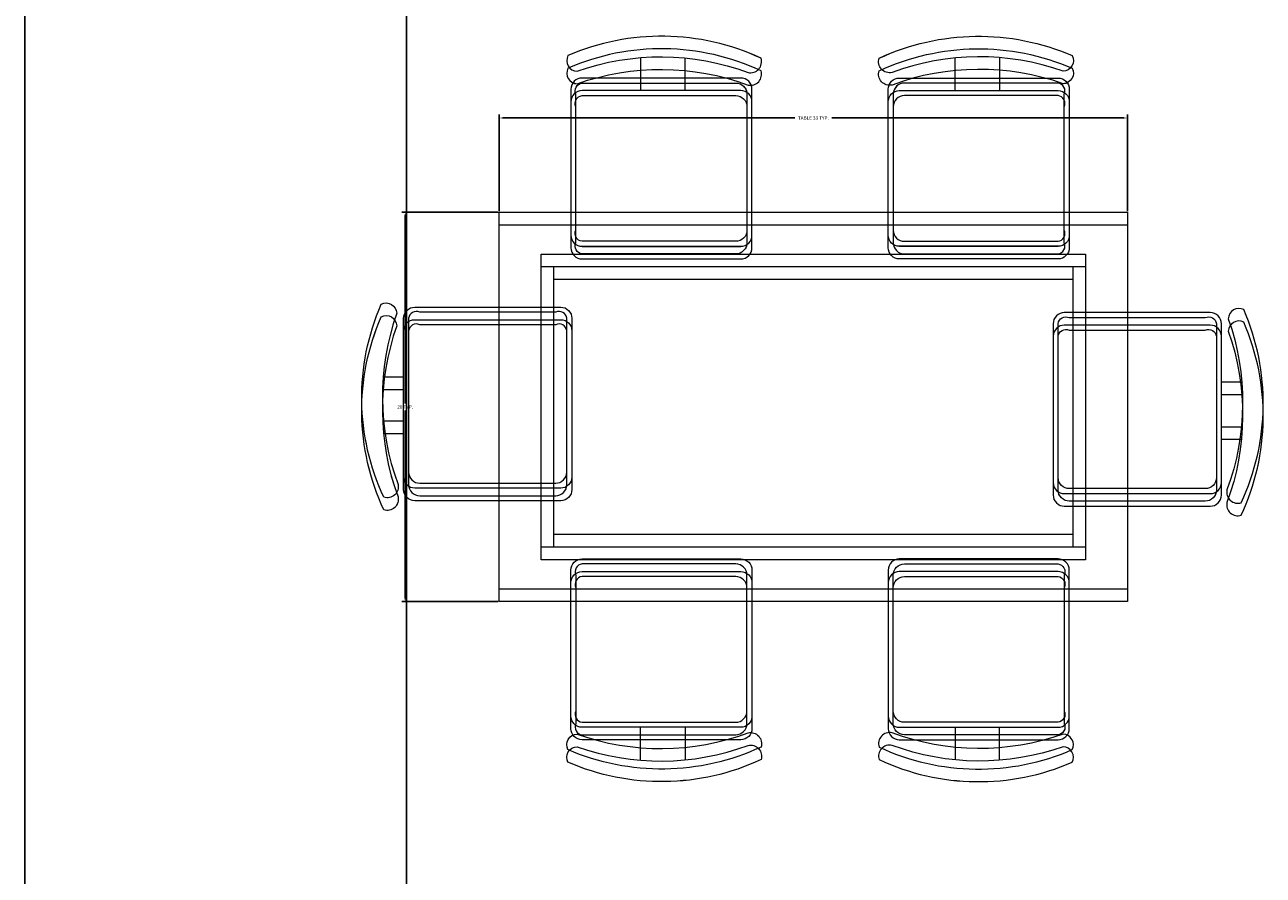
# Model space of a CAD drawing. Units: inches. Extents: x 1601 to 2297, y 1496 to 2631.
# Tile 52 of 57: x 2036 to 2100, y 2327 to 2371. Entities that reach past the tile are written whole.
import ezdxf

# ---------------------------------------------------------------- set-up
doc = ezdxf.new("R2010")
doc.units = ezdxf.units.IN
doc.layers.add('A-ANNO-DIMS', color=2, linetype='Continuous', lineweight=18)
doc.layers.add('A-FURN', color=8, linetype='Continuous', lineweight=18)
doc.styles.get("Standard").update_dxf_attribs({"font": 'arial.ttf'})
doc.dimstyles.get("Standard").update_dxf_attribs({"dimtxt": 0.18, "dimasz": 0.18, "dimexe": 0.18, "dimexo": 0.0625, "dimgap": 0.09, "dimtad": 0, "dimtih": 1, "dimtoh": 1, "dimdec": 4, "dimzin": 0, "dimdsep": 46, "dimtxsty": 'Standard', "dimcen": 0.09, "dimadec": 0, "dimazin": 0, "dimtfac": 1, "dimtdec": 4, "dimtofl": 0, "dimtmove": 0, "dimatfit": 3, "dimfxl": 1, "dimtolj": 1, "dimtzin": 0, "dimarcsym": 0})

# ---------------------------------------------------------------- blocks, each defined once
blk = doc.blocks.new('DINING-TABLE')
for points in [[(0, 20.416), (32.93, 20.416), (32.93, 0.659), (0, 0.659)], [(0, 20.416), (32.93, 20.416), (32.93, 0.658), (0, 0.658)], [(0, 20.416), (32.93, 20.416), (32.93, 0.659), (0, 0.659)], [(0, 20.416), (32.93, 20.416), (32.93, 0.658), (0, 0.658)], [(0, 19.758), (32.93, 19.758), (32.93, 0), (0, 0)], [(0, 19.758), (32.93, 19.758), (32.93, 0), (0, 0)], [(0, 19.758), (32.93, 19.758), (32.93, 0), (0, 0)], [(0, 19.758), (32.93, 19.758), (32.93, 0), (0, 0)], [(2.196, 18.221), (30.735, 18.221), (30.735, 2.854), (2.196, 2.854)], [(2.196, 18.221), (30.735, 18.221), (30.735, 2.854), (2.196, 2.854)], [(2.196, 18.221), (30.735, 18.221), (30.735, 2.854), (2.196, 2.854)], [(2.196, 18.221), (30.735, 18.221), (30.735, 2.854), (2.196, 2.854)], [(2.196, 17.563), (30.735, 17.563), (30.735, 2.195), (2.196, 2.195)], [(2.196, 17.563), (30.735, 17.563), (30.735, 2.195), (2.196, 2.195)], [(2.196, 17.562), (30.735, 17.562), (30.735, 2.195), (2.196, 2.195)], [(2.196, 17.562), (30.735, 17.562), (30.735, 2.195), (2.196, 2.195)], [(2.854, 17.563), (30.076, 17.563), (30.076, 3.513), (2.854, 3.513)], [(2.854, 17.563), (30.076, 17.563), (30.076, 3.513), (2.854, 3.513)], [(2.854, 17.562), (30.076, 17.562), (30.076, 3.512), (2.854, 3.512)], [(2.854, 17.562), (30.076, 17.562), (30.076, 3.512), (2.854, 3.512)], [(2.854, 16.904), (30.076, 16.904), (30.076, 2.854), (2.854, 2.854)], [(2.854, 16.904), (30.076, 16.904), (30.076, 2.854), (2.854, 2.854)], [(2.854, 16.904), (30.076, 16.904), (30.076, 2.854), (2.854, 2.854)], [(2.854, 16.904), (30.076, 16.904), (30.076, 2.854), (2.854, 2.854)]]:
    blk.add_lwpolyline(points, close=True)
blk = doc.blocks.new('*D16')
at = {"layer": 'A-ANNO-DIMS', "color": 0, "lineweight": -2, "transparency": 16777216}
for p, q in [((2060.42, 2361.732), (2060.42, 2366.789)), ((2060.6, 2366.609), (2075.922, 2366.609)), ((2093.17, 2366.609), (2077.849, 2366.609)), ((2093.35, 2361.732), (2093.35, 2366.789))]:
    blk.add_line(p, q, dxfattribs=at)
at = {"layer": 'A-ANNO-DIMS', "color": 0, "transparency": 16777216}
for points in [[(2060.6, 2366.639), (2060.6, 2366.579), (2060.42, 2366.609)], [(2093.17, 2366.639), (2093.17, 2366.579), (2093.35, 2366.609)]]:
    blk.add_solid(points, dxfattribs=at)
at = {"layer": 'Defpoints', "color": 0, "transparency": 16777216}
for p in [(2093.35, 2366.609), (2060.42, 2361.669), (2093.35, 2361.669)]:
    blk.add_point(p, dxfattribs=at)
at = {"layer": 'A-ANNO-DIMS', "color": 0, "transparency": 16777216, "insert": (2076.885, 2366.609), "char_height": 0.18, "attachment_point": 5}
blk.add_mtext('\\A1;TABLE 33 TYP.', dxfattribs=at)
blk = doc.blocks.new('*D17')
at = {"layer": 'A-ANNO-DIMS', "color": 0, "lineweight": -2, "transparency": 16777216}
for p, q in [((2060.358, 2361.669), (2055.301, 2361.669)), ((2055.481, 2361.489), (2055.481, 2351.643)), ((2055.481, 2341.433), (2055.481, 2351.279)), ((2060.358, 2341.253), (2055.301, 2341.253))]:
    blk.add_line(p, q, dxfattribs=at)
at = {"layer": 'A-ANNO-DIMS', "color": 0, "transparency": 16777216}
for points in [[(2055.451, 2361.489), (2055.511, 2361.489), (2055.481, 2361.669)], [(2055.451, 2341.433), (2055.511, 2341.433), (2055.481, 2341.253)]]:
    blk.add_solid(points, dxfattribs=at)
at = {"layer": 'Defpoints', "color": 0, "transparency": 16777216}
for p in [(2055.481, 2361.669), (2060.42, 2361.669), (2060.42, 2341.253)]:
    blk.add_point(p, dxfattribs=at)
at = {"layer": 'A-ANNO-DIMS', "color": 0, "transparency": 16777216, "insert": (2055.481, 2351.461), "char_height": 0.18, "attachment_point": 5}
blk.add_mtext('\\A1;20 TYP.', dxfattribs=at)
blk = doc.blocks.new('*D40')
at = {"layer": 'A-ANNO-DIMS', "color": 0, "lineweight": -2, "transparency": 16777216}
for p, q in [((2035.537, 1986.388), (2035.537, 2581.055)), ((2035.717, 2580.875), (2045.079, 2580.875)), ((2055.371, 2580.875), (2046.009, 2580.875)), ((2055.551, 1986.388), (2055.551, 2581.055))]:
    blk.add_line(p, q, dxfattribs=at)
at = {"layer": 'A-ANNO-DIMS', "color": 0, "transparency": 16777216}
for points in [[(2035.717, 2580.905), (2035.717, 2580.845), (2035.537, 2580.875)], [(2055.371, 2580.905), (2055.371, 2580.845), (2055.551, 2580.875)]]:
    blk.add_solid(points, dxfattribs=at)
at = {"layer": 'Defpoints', "color": 0, "transparency": 16777216}
for p in [(2055.551, 2580.875), (2035.537, 1986.325), (2055.551, 1986.325)]:
    blk.add_point(p, dxfattribs=at)
at = {"layer": 'A-ANNO-DIMS', "color": 0, "transparency": 16777216, "insert": (2045.544, 2580.875), "char_height": 0.18, "attachment_point": 5}
blk.add_mtext('\\A1;20.014', dxfattribs=at)

msp = doc.modelspace()

# ---------------------------------------------------------------- linework, layer by layer
at = {"layer": 'A-FURN'}
for points in [[(2064.4935, 2369.0615, -0.1758092), (2073.4626, 2368.9935, 0.5783921), (2074.1421, 2369.7407, 0.2145244), (2064.0179, 2369.8765, 0.552014), (2064.4935, 2369.0615, -0.065079)], [(2064.4935, 2369.0615, -0.1758092), (2073.4626, 2368.9935, 0.5783921), (2074.1421, 2369.7407, 0.2145244), (2064.0179, 2369.8765, 0.552014), (2064.4935, 2369.0615, -0.065079)], [(2064.4935, 2369.0611, -0.1758092), (2073.4626, 2368.9932, 0.5783921), (2074.1421, 2369.7403, 0.2145244), (2064.0179, 2369.8762, 0.552014), (2064.4935, 2369.0611, -0.065079)], [(2064.4935, 2369.0611, -0.1758092), (2073.4626, 2368.9932, 0.5783921), (2074.1421, 2369.7403, 0.2145244), (2064.0179, 2369.8762, 0.552014), (2064.4935, 2369.0611, -0.065079)], [(2081.0134, 2368.9935, -0.5783921), (2080.3339, 2369.7407, -0.2145244), (2090.4581, 2369.8765, -0.552014), (2089.9825, 2369.0615, 0.1758092), (2081.0134, 2368.9935)], [(2081.0134, 2368.9935, -0.5783921), (2080.3339, 2369.7407, -0.2145244), (2090.4581, 2369.8765, -0.552014), (2089.9825, 2369.0615, 0.1758092), (2081.0134, 2368.9935)], [(2081.0134, 2368.9932, -0.5783921), (2080.334, 2369.7403, -0.2145244), (2090.4582, 2369.8762, -0.552014), (2089.9825, 2369.0611, 0.1758092), (2081.0134, 2368.9932)], [(2081.0134, 2368.9932, -0.5783921), (2080.334, 2369.7403, -0.2145244), (2090.4582, 2369.8762, -0.552014), (2089.9825, 2369.0611, 0.1758092), (2081.0134, 2368.9932)], [(2064.4935, 2368.4029, -0.1758092), (2073.4626, 2368.3349, 0.5783921), (2074.1421, 2369.0821, 0.2145244), (2064.0179, 2369.2179, 0.552014), (2064.4935, 2368.4029, -0.065079)], [(2064.4935, 2368.4029, -0.1758092), (2073.4626, 2368.3349, 0.5783921), (2074.1421, 2369.0821, 0.2145244), (2064.0179, 2369.2179, 0.552014), (2064.4935, 2368.4029, -0.065079)], [(2064.4935, 2368.4025, -0.1758092), (2073.4626, 2368.3346, 0.5783921), (2074.1421, 2369.0817, 0.2145244), (2064.0179, 2369.2176, 0.552014), (2064.4935, 2368.4025, -0.065079)], [(2064.4935, 2368.4025, -0.1758092), (2073.4626, 2368.3346, 0.5783921), (2074.1421, 2369.0817, 0.2145244), (2064.0179, 2369.2176, 0.552014), (2064.4935, 2368.4025, -0.065079)], [(2081.0134, 2368.3349, -0.5783921), (2080.3339, 2369.0821, -0.2145244), (2090.4581, 2369.2179, -0.552014), (2089.9825, 2368.4029, 0.1758092), (2081.0134, 2368.3349)], [(2081.0134, 2368.3349, -0.5783921), (2080.3339, 2369.0821, -0.2145244), (2090.4581, 2369.2179, -0.552014), (2089.9825, 2368.4029, 0.1758092), (2081.0134, 2368.3349)], [(2081.0134, 2368.3346, -0.5783921), (2080.334, 2369.0817, -0.2145244), (2090.4582, 2369.2176, -0.552014), (2089.9825, 2368.4025, 0.1758092), (2081.0134, 2368.3346)], [(2081.0134, 2368.3346, -0.5783921), (2080.334, 2369.0817, -0.2145244), (2090.4582, 2369.2176, -0.552014), (2089.9825, 2368.4025, 0.1758092), (2081.0134, 2368.3346)], [(2070.1574, 2368.7015), (2070.1574, 2369.7545, -0.0647586)], [(2070.1574, 2368.7015), (2070.1574, 2369.7545, -0.0647586)], [(2070.1574, 2368.7011), (2070.1574, 2369.7542, -0.0647586)], [(2070.1574, 2368.7011), (2070.1574, 2369.7542, -0.0647586)], [(2084.3187, 2368.7015), (2084.3187, 2369.7545, 0.0647586)], [(2084.3187, 2368.7015), (2084.3187, 2369.7545, 0.0647586)], [(2084.3187, 2368.7011), (2084.3187, 2369.7542, 0.0647586)], [(2084.3187, 2368.7011), (2084.3187, 2369.7542, 0.0647586)], [(2070.1574, 2368.0429), (2070.1574, 2369.0959, -0.0647586)], [(2070.1574, 2368.0429), (2070.1574, 2369.0959, -0.0647586)], [(2070.1574, 2368.0425), (2070.1574, 2369.0956, -0.0647586)], [(2070.1574, 2368.0425), (2070.1574, 2369.0956, -0.0647586)], [(2084.3187, 2368.0429), (2084.3187, 2369.0959, 0.0647586)], [(2084.3187, 2368.0429), (2084.3187, 2369.0959, 0.0647586)], [(2084.3187, 2368.0425), (2084.3187, 2369.0956, 0.0647586)], [(2084.3187, 2368.0425), (2084.3187, 2369.0956, 0.0647586)], [(2073.0821, 2368.7015), (2064.7555, 2368.7015, 0.4142136), (2064.173, 2368.1189), (2064.173, 2360.4628, 0.4142136), (2064.7555, 2359.8803), (2073.0821, 2359.8803, 0.4142136), (2073.6646, 2360.4628), (2073.6646, 2368.1189, 0.4142136), (2073.0821, 2368.7015)], [(2073.0821, 2368.7015), (2064.7555, 2368.7015, 0.4142136), (2064.173, 2368.1189), (2064.173, 2360.4628, 0.4142136), (2064.7555, 2359.8803), (2073.0821, 2359.8803, 0.4142136), (2073.6646, 2360.4628), (2073.6646, 2368.1189, 0.4142136), (2073.0821, 2368.7015)], [(2073.0821, 2368.7011), (2064.7555, 2368.7011, 0.4142136), (2064.173, 2368.1186), (2064.173, 2360.4625, 0.4142136), (2064.7555, 2359.8799), (2073.0821, 2359.8799, 0.4142136), (2073.6646, 2360.4625), (2073.6646, 2368.1186, 0.4142136), (2073.0821, 2368.7011)], [(2073.0821, 2368.7011), (2064.7555, 2368.7011, 0.4142136), (2064.173, 2368.1186), (2064.173, 2360.4625, 0.4142136), (2064.7555, 2359.8799), (2073.0821, 2359.8799, 0.4142136), (2073.6646, 2360.4625), (2073.6646, 2368.1186, 0.4142136), (2073.0821, 2368.7011)], [(2089.7205, 2368.7015, -0.4142136), (2090.3031, 2368.1189), (2090.3031, 2360.4628, -0.4142136), (2089.7205, 2359.8803), (2081.3939, 2359.8803, -0.4142136), (2080.8114, 2360.4628), (2080.8114, 2368.1189, -0.4142136), (2081.3939, 2368.7015), (2089.7205, 2368.7015)], [(2089.7205, 2368.7015, -0.4142136), (2090.3031, 2368.1189), (2090.3031, 2360.4628, -0.4142136), (2089.7205, 2359.8803), (2081.3939, 2359.8803, -0.4142136), (2080.8114, 2360.4628), (2080.8114, 2368.1189, -0.4142136), (2081.3939, 2368.7015), (2089.7205, 2368.7015)], [(2089.7205, 2368.7011, -0.4142136), (2090.3031, 2368.1186), (2090.3031, 2360.4625, -0.4142136), (2089.7205, 2359.8799), (2081.394, 2359.8799, -0.4142136), (2080.8114, 2360.4625), (2080.8114, 2368.1186, -0.4142136), (2081.394, 2368.7011), (2089.7205, 2368.7011)], [(2089.7205, 2368.7011, -0.4142136), (2090.3031, 2368.1186), (2090.3031, 2360.4625, -0.4142136), (2089.7205, 2359.8799), (2081.394, 2359.8799, -0.4142136), (2080.8114, 2360.4625), (2080.8114, 2368.1186, -0.4142136), (2081.394, 2368.7011), (2089.7205, 2368.7011)], [(2073.0821, 2368.0429), (2064.7555, 2368.0429, 0.4142136), (2064.173, 2367.4604), (2064.173, 2359.8042, 0.4142136), (2064.7555, 2359.2217), (2073.0821, 2359.2217, 0.4142136), (2073.6646, 2359.8042), (2073.6646, 2367.4604, 0.4142136), (2073.0821, 2368.0429)], [(2073.0821, 2368.0429), (2064.7555, 2368.0429, 0.4142136), (2064.173, 2367.4604), (2064.173, 2359.8042, 0.4142136), (2064.7555, 2359.2217), (2073.0821, 2359.2217, 0.4142136), (2073.6646, 2359.8042), (2073.6646, 2367.4604, 0.4142136), (2073.0821, 2368.0429)], [(2073.0821, 2368.0425), (2064.7555, 2368.0425, 0.4142136), (2064.173, 2367.46), (2064.173, 2359.8039, 0.4142136), (2064.7555, 2359.2213), (2073.0821, 2359.2213, 0.4142136), (2073.6646, 2359.8039), (2073.6646, 2367.46, 0.4142136), (2073.0821, 2368.0425)], [(2073.0821, 2368.0425), (2064.7555, 2368.0425, 0.4142136), (2064.173, 2367.46), (2064.173, 2359.8039, 0.4142136), (2064.7555, 2359.2213), (2073.0821, 2359.2213, 0.4142136), (2073.6646, 2359.8039), (2073.6646, 2367.46, 0.4142136), (2073.0821, 2368.0425)], [(2089.7205, 2368.0429, -0.4142136), (2090.3031, 2367.4604), (2090.3031, 2359.8042, -0.4142136), (2089.7205, 2359.2217), (2081.3939, 2359.2217, -0.4142136), (2080.8114, 2359.8042), (2080.8114, 2367.4604, -0.4142136), (2081.3939, 2368.0429), (2089.7205, 2368.0429)], [(2089.7205, 2368.0429, -0.4142136), (2090.3031, 2367.4604), (2090.3031, 2359.8042, -0.4142136), (2089.7205, 2359.2217), (2081.3939, 2359.2217, -0.4142136), (2080.8114, 2359.8042), (2080.8114, 2367.4604, -0.4142136), (2081.3939, 2368.0429), (2089.7205, 2368.0429)], [(2089.7205, 2368.0425, -0.4142136), (2090.3031, 2367.46), (2090.3031, 2359.8039, -0.4142136), (2089.7205, 2359.2213), (2081.394, 2359.2213, -0.4142136), (2080.8114, 2359.8039), (2080.8114, 2367.46, -0.4142136), (2081.394, 2368.0425), (2089.7205, 2368.0425)], [(2089.7205, 2368.0425, -0.4142136), (2090.3031, 2367.46), (2090.3031, 2359.8039, -0.4142136), (2089.7205, 2359.2213), (2081.394, 2359.2213, -0.4142136), (2080.8114, 2359.8039), (2080.8114, 2367.46, -0.4142136), (2081.394, 2368.0425), (2089.7205, 2368.0425)], [(2055.1101, 2347.4025, -0.5783921), (2054.363, 2346.723, -0.2145244), (2054.2272, 2356.8472, -0.552014), (2055.0422, 2356.3716, 0.1758094), (2055.1101, 2347.4025)], [(2055.1101, 2347.4025, -0.5783921), (2054.363, 2346.723, -0.2145244), (2054.2272, 2356.8472, -0.552014), (2055.0422, 2356.3716, 0.1758094), (2055.1101, 2347.4025)], [(2055.1102, 2347.4021, -0.5783921), (2054.363, 2346.7227, -0.2145244), (2054.2272, 2356.8469, -0.552014), (2055.0422, 2356.3712, 0.1758094), (2055.1102, 2347.4021)], [(2055.1102, 2347.4021, -0.5783921), (2054.363, 2346.7227, -0.2145244), (2054.2272, 2356.8469, -0.552014), (2055.0422, 2356.3712, 0.1758094), (2055.1102, 2347.4021)], [(2055.4022, 2356.1096, -0.4142136), (2055.9847, 2356.6921), (2063.6409, 2356.6921, -0.4142136), (2064.2234, 2356.1096), (2064.2234, 2347.783, -0.4142136), (2063.6409, 2347.2005), (2055.9847, 2347.2005, -0.4142136), (2055.4022, 2347.783), (2055.4022, 2356.1096)], [(2055.4022, 2356.1096, -0.4142136), (2055.9847, 2356.6921), (2063.6409, 2356.6921, -0.4142136), (2064.2234, 2356.1096), (2064.2234, 2347.783, -0.4142136), (2063.6409, 2347.2005), (2055.9847, 2347.2005, -0.4142136), (2055.4022, 2347.783), (2055.4022, 2356.1096)], [(2055.4022, 2356.1093, -0.4142136), (2055.9848, 2356.6918), (2063.6409, 2356.6918, -0.4142136), (2064.2234, 2356.1093), (2064.2234, 2347.7827, -0.4142136), (2063.6409, 2347.2001), (2055.9848, 2347.2001, -0.4142136), (2055.4022, 2347.7827), (2055.4022, 2356.1093)], [(2055.4022, 2356.1093, -0.4142136), (2055.9848, 2356.6918), (2063.6409, 2356.6918, -0.4142136), (2064.2234, 2356.1093), (2064.2234, 2347.7827, -0.4142136), (2063.6409, 2347.2001), (2055.9848, 2347.2001, -0.4142136), (2055.4022, 2347.7827), (2055.4022, 2356.1093)], [(2098.6402, 2356.0864, -0.1758092), (2098.5723, 2347.1173, 0.5783921), (2099.3195, 2346.4378, 0.2145244), (2099.4553, 2356.562, 0.552014), (2098.6402, 2356.0864, -0.065079)], [(2098.6402, 2356.0864, -0.1758092), (2098.5723, 2347.1173, 0.5783921), (2099.3195, 2346.4378, 0.2145244), (2099.4553, 2356.562, 0.552014), (2098.6402, 2356.0864, -0.065079)], [(2098.6403, 2356.086, -0.1758092), (2098.5723, 2347.117, 0.5783921), (2099.3195, 2346.4375, 0.2145244), (2099.4553, 2356.5617, 0.552014), (2098.6403, 2356.0861, -0.065079)], [(2098.6403, 2356.086, -0.1758092), (2098.5723, 2347.117, 0.5783921), (2099.3195, 2346.4375, 0.2145244), (2099.4553, 2356.5617, 0.552014), (2098.6403, 2356.0861, -0.065079)], [(2055.1101, 2346.7439, -0.5783921), (2054.363, 2346.0644, -0.2145244), (2054.2272, 2356.1886, -0.552014), (2055.0422, 2355.713, 0.1758094), (2055.1101, 2346.7439)], [(2055.1101, 2346.7439, -0.5783921), (2054.363, 2346.0644, -0.2145244), (2054.2272, 2356.1886, -0.552014), (2055.0422, 2355.713, 0.1758094), (2055.1101, 2346.7439)], [(2055.1102, 2346.7435, -0.5783921), (2054.363, 2346.0641, -0.2145244), (2054.2272, 2356.1883, -0.552014), (2055.0422, 2355.7126, 0.1758094), (2055.1102, 2346.7435)], [(2055.1102, 2346.7435, -0.5783921), (2054.363, 2346.0641, -0.2145244), (2054.2272, 2356.1883, -0.552014), (2055.0422, 2355.7126, 0.1758094), (2055.1102, 2346.7435)], [(2055.4022, 2355.451, -0.4142136), (2055.9847, 2356.0335), (2063.6409, 2356.0335, -0.4142136), (2064.2234, 2355.451), (2064.2234, 2347.1244, -0.4142136), (2063.6409, 2346.5419), (2055.9847, 2346.5419, -0.4142136), (2055.4022, 2347.1244), (2055.4022, 2355.451)], [(2055.4022, 2355.451, -0.4142136), (2055.9847, 2356.0335), (2063.6409, 2356.0335, -0.4142136), (2064.2234, 2355.451), (2064.2234, 2347.1244, -0.4142136), (2063.6409, 2346.5419), (2055.9847, 2346.5419, -0.4142136), (2055.4022, 2347.1244), (2055.4022, 2355.451)], [(2055.4022, 2355.4507, -0.4142136), (2055.9848, 2356.0332), (2063.6409, 2356.0332, -0.4142136), (2064.2234, 2355.4507), (2064.2234, 2347.1241, -0.4142136), (2063.6409, 2346.5415), (2055.9848, 2346.5415, -0.4142136), (2055.4022, 2347.1241), (2055.4022, 2355.4507)], [(2055.4022, 2355.4507, -0.4142136), (2055.9848, 2356.0332), (2063.6409, 2356.0332, -0.4142136), (2064.2234, 2355.4507), (2064.2234, 2347.1241, -0.4142136), (2063.6409, 2346.5415), (2055.9848, 2346.5415, -0.4142136), (2055.4022, 2347.1241), (2055.4022, 2355.4507)], [(2098.2803, 2355.8244, 0.4142136), (2097.6977, 2356.407), (2090.0416, 2356.407, 0.4142136), (2089.459, 2355.8244), (2089.459, 2347.4978, 0.4142136), (2090.0416, 2346.9153), (2097.6977, 2346.9153, 0.4142136), (2098.2803, 2347.4978), (2098.2803, 2355.8244)], [(2098.2803, 2355.8244, 0.4142136), (2097.6977, 2356.407), (2090.0416, 2356.407, 0.4142136), (2089.459, 2355.8244), (2089.459, 2347.4978, 0.4142136), (2090.0416, 2346.9153), (2097.6977, 2346.9153, 0.4142136), (2098.2803, 2347.4978), (2098.2803, 2355.8244)], [(2098.2803, 2355.8241, 0.4142136), (2097.6977, 2356.4066), (2090.0416, 2356.4066, 0.4142136), (2089.4591, 2355.8241), (2089.4591, 2347.4975, 0.4142136), (2090.0416, 2346.915), (2097.6977, 2346.915, 0.4142136), (2098.2803, 2347.4975), (2098.2803, 2355.8241)], [(2098.2803, 2355.8241, 0.4142136), (2097.6977, 2356.4066), (2090.0416, 2356.4066, 0.4142136), (2089.4591, 2355.8241), (2089.4591, 2347.4975, 0.4142136), (2090.0416, 2346.915), (2097.6977, 2346.915, 0.4142136), (2098.2803, 2347.4975), (2098.2803, 2355.8241)], [(2098.6402, 2355.4278, -0.1758092), (2098.5723, 2346.4587, 0.5783921), (2099.3195, 2345.7792, 0.2145244), (2099.4553, 2355.9034, 0.552014), (2098.6402, 2355.4278, -0.065079)], [(2098.6402, 2355.4278, -0.1758092), (2098.5723, 2346.4587, 0.5783921), (2099.3195, 2345.7792, 0.2145244), (2099.4553, 2355.9034, 0.552014), (2098.6402, 2355.4278, -0.065079)], [(2098.6403, 2355.4275, -0.1758092), (2098.5723, 2346.4584, 0.5783921), (2099.3195, 2345.7789, 0.2145244), (2099.4553, 2355.9031, 0.552014), (2098.6403, 2355.4275, -0.065079)], [(2098.6403, 2355.4275, -0.1758092), (2098.5723, 2346.4584, 0.5783921), (2099.3195, 2345.7789, 0.2145244), (2099.4553, 2355.9031, 0.552014), (2098.6403, 2355.4275, -0.065079)], [(2098.2803, 2355.1658, 0.4142136), (2097.6977, 2355.7484), (2090.0416, 2355.7484, 0.4142136), (2089.459, 2355.1658), (2089.459, 2346.8392, 0.4142136), (2090.0416, 2346.2567), (2097.6977, 2346.2567, 0.4142136), (2098.2803, 2346.8392), (2098.2803, 2355.1658)], [(2098.2803, 2355.1658, 0.4142136), (2097.6977, 2355.7484), (2090.0416, 2355.7484, 0.4142136), (2089.459, 2355.1658), (2089.459, 2346.8392, 0.4142136), (2090.0416, 2346.2567), (2097.6977, 2346.2567, 0.4142136), (2098.2803, 2346.8392), (2098.2803, 2355.1658)], [(2098.2803, 2355.1655, 0.4142136), (2097.6977, 2355.748), (2090.0416, 2355.748, 0.4142136), (2089.4591, 2355.1655), (2089.4591, 2346.8389, 0.4142136), (2090.0416, 2346.2564), (2097.6977, 2346.2564, 0.4142136), (2098.2803, 2346.8389), (2098.2803, 2355.1655)], [(2098.2803, 2355.1655, 0.4142136), (2097.6977, 2355.748), (2090.0416, 2355.748, 0.4142136), (2089.4591, 2355.1655), (2089.4591, 2346.8389, 0.4142136), (2090.0416, 2346.2564), (2097.6977, 2346.2564, 0.4142136), (2098.2803, 2346.8389), (2098.2803, 2355.1655)], [(2055.4022, 2350.7077), (2054.3491, 2350.7077, 0.0647586)], [(2055.4022, 2350.7077), (2054.3491, 2350.7077, 0.0647586)], [(2055.4022, 2350.7074), (2054.3492, 2350.7074, 0.0647586)], [(2055.4022, 2350.7074), (2054.3492, 2350.7074, 0.0647586)], [(2098.2803, 2350.4226), (2099.3333, 2350.4226, -0.0647586)], [(2098.2803, 2350.4226), (2099.3333, 2350.4226, -0.0647586)], [(2098.2803, 2350.4222), (2099.3333, 2350.4222, -0.0647586)], [(2098.2803, 2350.4222), (2099.3333, 2350.4222, -0.0647586)], [(2055.4022, 2350.0491), (2054.3491, 2350.0491, 0.0647586)], [(2055.4022, 2350.0491), (2054.3491, 2350.0491, 0.0647586)], [(2055.4022, 2350.0488), (2054.3492, 2350.0488, 0.0647586)], [(2055.4022, 2350.0488), (2054.3492, 2350.0488, 0.0647586)], [(2098.2803, 2349.764), (2099.3333, 2349.764, -0.0647586)], [(2098.2803, 2349.764), (2099.3333, 2349.764, -0.0647586)], [(2098.2803, 2349.7636), (2099.3333, 2349.7636, -0.0647586)], [(2098.2803, 2349.7636), (2099.3333, 2349.7636, -0.0647586)], [(2073.0821, 2334.6681), (2064.7555, 2334.6681, -0.4142136), (2064.173, 2335.2506), (2064.173, 2342.9067, -0.4142136), (2064.7555, 2343.4893), (2073.0821, 2343.4893, -0.4142136), (2073.6646, 2342.9067), (2073.6646, 2335.2506, -0.4142136), (2073.0821, 2334.6681)], [(2073.0821, 2334.6681), (2064.7555, 2334.6681, -0.4142136), (2064.173, 2335.2506), (2064.173, 2342.9067, -0.4142136), (2064.7555, 2343.4893), (2073.0821, 2343.4893, -0.4142136), (2073.6646, 2342.9067), (2073.6646, 2335.2506, -0.4142136), (2073.0821, 2334.6681)], [(2073.0821, 2334.6677), (2064.7555, 2334.6677, -0.4142136), (2064.173, 2335.2502), (2064.173, 2342.9064, -0.4142136), (2064.7555, 2343.4889), (2073.0821, 2343.4889, -0.4142136), (2073.6646, 2342.9064), (2073.6646, 2335.2502, -0.4142136), (2073.0821, 2334.6677)], [(2073.0821, 2334.6677), (2064.7555, 2334.6677, -0.4142136), (2064.173, 2335.2502), (2064.173, 2342.9064, -0.4142136), (2064.7555, 2343.4889), (2073.0821, 2343.4889, -0.4142136), (2073.6646, 2342.9064), (2073.6646, 2335.2502, -0.4142136), (2073.0821, 2334.6677)], [(2089.7205, 2334.6681, 0.4142136), (2090.3031, 2335.2506), (2090.3031, 2342.9067, 0.4142136), (2089.7205, 2343.4893), (2081.3939, 2343.4893, 0.4142136), (2080.8114, 2342.9067), (2080.8114, 2335.2506, 0.4142136), (2081.3939, 2334.6681), (2089.7205, 2334.6681)], [(2089.7205, 2334.6681, 0.4142136), (2090.3031, 2335.2506), (2090.3031, 2342.9067, 0.4142136), (2089.7205, 2343.4893), (2081.3939, 2343.4893, 0.4142136), (2080.8114, 2342.9067), (2080.8114, 2335.2506, 0.4142136), (2081.3939, 2334.6681), (2089.7205, 2334.6681)], [(2089.7205, 2334.6677, 0.4142136), (2090.3031, 2335.2502), (2090.3031, 2342.9064, 0.4142136), (2089.7205, 2343.4889), (2081.394, 2343.4889, 0.4142136), (2080.8114, 2342.9064), (2080.8114, 2335.2502, 0.4142136), (2081.394, 2334.6677), (2089.7205, 2334.6677)], [(2089.7205, 2334.6677, 0.4142136), (2090.3031, 2335.2502), (2090.3031, 2342.9064, 0.4142136), (2089.7205, 2343.4889), (2081.394, 2343.4889, 0.4142136), (2080.8114, 2342.9064), (2080.8114, 2335.2502, 0.4142136), (2081.394, 2334.6677), (2089.7205, 2334.6677)], [(2073.0821, 2334.0095), (2064.7555, 2334.0095, -0.4142136), (2064.173, 2334.592), (2064.173, 2342.2481, -0.4142136), (2064.7555, 2342.8307), (2073.0821, 2342.8307, -0.4142136), (2073.6646, 2342.2481), (2073.6646, 2334.592, -0.4142136), (2073.0821, 2334.0095)], [(2073.0821, 2334.0095), (2064.7555, 2334.0095, -0.4142136), (2064.173, 2334.592), (2064.173, 2342.2481, -0.4142136), (2064.7555, 2342.8307), (2073.0821, 2342.8307, -0.4142136), (2073.6646, 2342.2481), (2073.6646, 2334.592, -0.4142136), (2073.0821, 2334.0095)], [(2073.0821, 2334.0091), (2064.7555, 2334.0091, -0.4142136), (2064.173, 2334.5917), (2064.173, 2342.2478, -0.4142136), (2064.7555, 2342.8303), (2073.0821, 2342.8303, -0.4142136), (2073.6646, 2342.2478), (2073.6646, 2334.5917, -0.4142136), (2073.0821, 2334.0091)], [(2073.0821, 2334.0091), (2064.7555, 2334.0091, -0.4142136), (2064.173, 2334.5917), (2064.173, 2342.2478, -0.4142136), (2064.7555, 2342.8303), (2073.0821, 2342.8303, -0.4142136), (2073.6646, 2342.2478), (2073.6646, 2334.5917, -0.4142136), (2073.0821, 2334.0091)], [(2089.7205, 2334.0095, 0.4142136), (2090.3031, 2334.592), (2090.3031, 2342.2481, 0.4142136), (2089.7205, 2342.8307), (2081.3939, 2342.8307, 0.4142136), (2080.8114, 2342.2481), (2080.8114, 2334.592, 0.4142136), (2081.3939, 2334.0095), (2089.7205, 2334.0095)], [(2089.7205, 2334.0095, 0.4142136), (2090.3031, 2334.592), (2090.3031, 2342.2481, 0.4142136), (2089.7205, 2342.8307), (2081.3939, 2342.8307, 0.4142136), (2080.8114, 2342.2481), (2080.8114, 2334.592, 0.4142136), (2081.3939, 2334.0095), (2089.7205, 2334.0095)], [(2089.7205, 2334.0091, 0.4142136), (2090.3031, 2334.5917), (2090.3031, 2342.2478, 0.4142136), (2089.7205, 2342.8303), (2081.394, 2342.8303, 0.4142136), (2080.8114, 2342.2478), (2080.8114, 2334.5917, 0.4142136), (2081.394, 2334.0091), (2089.7205, 2334.0091)], [(2089.7205, 2334.0091, 0.4142136), (2090.3031, 2334.5917), (2090.3031, 2342.2478, 0.4142136), (2089.7205, 2342.8303), (2081.394, 2342.8303, 0.4142136), (2080.8114, 2342.2478), (2080.8114, 2334.5917, 0.4142136), (2081.394, 2334.0091), (2089.7205, 2334.0091)], [(2070.1574, 2334.6681), (2070.1574, 2333.615, 0.0647586)], [(2070.1574, 2334.6681), (2070.1574, 2333.615, 0.0647586)], [(2070.1574, 2334.6677), (2070.1574, 2333.6147, 0.0647586)], [(2070.1574, 2334.6677), (2070.1574, 2333.6147, 0.0647586)], [(2084.3187, 2334.6681), (2084.3187, 2333.615, -0.0647586)], [(2084.3187, 2334.6681), (2084.3187, 2333.615, -0.0647586)], [(2084.3187, 2334.6677), (2084.3187, 2333.6147, -0.0647586)], [(2084.3187, 2334.6677), (2084.3187, 2333.6147, -0.0647586)], [(2073.4626, 2334.376, -0.5783921), (2074.1421, 2333.6289, -0.2145244), (2064.0179, 2333.493, -0.552014), (2064.4935, 2334.3081, 0.1758093), (2073.4626, 2334.376)], [(2073.4626, 2334.376, -0.5783921), (2074.1421, 2333.6289, -0.2145244), (2064.0179, 2333.493, -0.552014), (2064.4935, 2334.3081, 0.1758093), (2073.4626, 2334.376)], [(2073.4626, 2334.3757, -0.5783921), (2074.1421, 2333.6285, -0.2145244), (2064.0179, 2333.4927, -0.552014), (2064.4935, 2334.3077, 0.1758093), (2073.4626, 2334.3757)], [(2073.4626, 2334.3757, -0.5783921), (2074.1421, 2333.6285, -0.2145244), (2064.0179, 2333.4927, -0.552014), (2064.4935, 2334.3077, 0.1758093), (2073.4626, 2334.3757)], [(2070.1574, 2334.0095), (2070.1574, 2332.9564, 0.0647586)], [(2070.1574, 2334.0095), (2070.1574, 2332.9564, 0.0647586)], [(2070.1574, 2334.0091), (2070.1574, 2332.9561, 0.0647586)], [(2070.1574, 2334.0091), (2070.1574, 2332.9561, 0.0647586)], [(2089.9825, 2334.3081, -0.1758093), (2081.0134, 2334.376, 0.5783921), (2080.3339, 2333.6289, 0.2145244), (2090.4581, 2333.493, 0.552014), (2089.9825, 2334.3081, -0.065079)], [(2089.9825, 2334.3081, -0.1758093), (2081.0134, 2334.376, 0.5783921), (2080.3339, 2333.6289, 0.2145244), (2090.4581, 2333.493, 0.552014), (2089.9825, 2334.3081, -0.065079)], [(2089.9825, 2334.3077, -0.1758093), (2081.0134, 2334.3757, 0.5783921), (2080.334, 2333.6285, 0.2145244), (2090.4582, 2333.4927, 0.552014), (2089.9825, 2334.3077, -0.065079)], [(2089.9825, 2334.3077, -0.1758093), (2081.0134, 2334.3757, 0.5783921), (2080.334, 2333.6285, 0.2145244), (2090.4582, 2333.4927, 0.552014), (2089.9825, 2334.3077, -0.065079)], [(2084.3187, 2334.0095), (2084.3187, 2332.9564, -0.0647586)], [(2084.3187, 2334.0095), (2084.3187, 2332.9564, -0.0647586)], [(2084.3187, 2334.0091), (2084.3187, 2332.9561, -0.0647586)], [(2084.3187, 2334.0091), (2084.3187, 2332.9561, -0.0647586)], [(2073.4626, 2333.7174, -0.5783921), (2074.1421, 2332.9703, -0.2145244), (2064.0179, 2332.8344, -0.552014), (2064.4935, 2333.6495, 0.1758093), (2073.4626, 2333.7174)], [(2073.4626, 2333.7174, -0.5783921), (2074.1421, 2332.9703, -0.2145244), (2064.0179, 2332.8344, -0.552014), (2064.4935, 2333.6495, 0.1758093), (2073.4626, 2333.7174)], [(2073.4626, 2333.7171, -0.5783921), (2074.1421, 2332.9699, -0.2145244), (2064.0179, 2332.8341, -0.552014), (2064.4935, 2333.6491, 0.1758093), (2073.4626, 2333.7171)], [(2073.4626, 2333.7171, -0.5783921), (2074.1421, 2332.9699, -0.2145244), (2064.0179, 2332.8341, -0.552014), (2064.4935, 2333.6491, 0.1758093), (2073.4626, 2333.7171)], [(2089.9825, 2333.6495, -0.1758093), (2081.0134, 2333.7174, 0.5783921), (2080.3339, 2332.9703, 0.2145244), (2090.4581, 2332.8344, 0.552014), (2089.9825, 2333.6495, -0.065079)], [(2089.9825, 2333.6495, -0.1758093), (2081.0134, 2333.7174, 0.5783921), (2080.3339, 2332.9703, 0.2145244), (2090.4581, 2332.8344, 0.552014), (2089.9825, 2333.6495, -0.065079)], [(2089.9825, 2333.6491, -0.1758093), (2081.0134, 2333.7171, 0.5783921), (2080.334, 2332.9699, 0.2145244), (2090.4582, 2332.8341, 0.552014), (2089.9825, 2333.6491, -0.065079)], [(2089.9825, 2333.6491, -0.1758093), (2081.0134, 2333.7171, 0.5783921), (2080.334, 2332.9699, 0.2145244), (2090.4582, 2332.8341, 0.552014), (2089.9825, 2333.6491, -0.065079)]]:
    msp.add_lwpolyline(points, format="xyb", dxfattribs=at)
for points in [[(2067.8266, 2369.7737), (2067.8266, 2368.7015)], [(2067.8266, 2369.7737), (2067.8266, 2368.7015)], [(2067.8267, 2369.7733), (2067.8267, 2368.7011)], [(2067.8267, 2369.7733), (2067.8267, 2368.7011)], [(2086.6494, 2369.7737), (2086.6494, 2368.7015)], [(2086.6494, 2369.7737), (2086.6494, 2368.7015)], [(2086.6494, 2369.7733), (2086.6494, 2368.7011)], [(2086.6494, 2369.7733), (2086.6494, 2368.7011)], [(2067.8266, 2369.1151), (2067.8266, 2368.0429)], [(2067.8266, 2369.1151), (2067.8266, 2368.0429)], [(2067.8267, 2369.1147), (2067.8267, 2368.0425)], [(2067.8267, 2369.1147), (2067.8267, 2368.0425)], [(2086.6494, 2369.1151), (2086.6494, 2368.0429)], [(2086.6494, 2369.1151), (2086.6494, 2368.0429)], [(2086.6494, 2369.1147), (2086.6494, 2368.0425)], [(2086.6494, 2369.1147), (2086.6494, 2368.0425)], [(2054.33, 2353.0385), (2055.4022, 2353.0385)], [(2054.33, 2353.0385), (2055.4022, 2353.0385)], [(2054.33, 2353.0381), (2055.4022, 2353.0381)], [(2054.33, 2353.0381), (2055.4022, 2353.0381)], [(2099.3525, 2352.7533), (2098.2803, 2352.7533)], [(2099.3525, 2352.7533), (2098.2803, 2352.7533)], [(2099.3525, 2352.7529), (2098.2803, 2352.7529)], [(2099.3525, 2352.7529), (2098.2803, 2352.7529)], [(2054.33, 2352.3799), (2055.4022, 2352.3799)], [(2054.33, 2352.3799), (2055.4022, 2352.3799)], [(2054.33, 2352.3795), (2055.4022, 2352.3795)], [(2054.33, 2352.3795), (2055.4022, 2352.3795)], [(2099.3525, 2352.0947), (2098.2803, 2352.0947)], [(2099.3525, 2352.0947), (2098.2803, 2352.0947)], [(2099.3525, 2352.0944), (2098.2803, 2352.0944)], [(2099.3525, 2352.0944), (2098.2803, 2352.0944)], [(2067.8266, 2333.5959), (2067.8266, 2334.6681)], [(2067.8266, 2333.5959), (2067.8266, 2334.6681)], [(2067.8267, 2333.5955), (2067.8267, 2334.6677)], [(2067.8267, 2333.5955), (2067.8267, 2334.6677)], [(2086.6494, 2333.5959), (2086.6494, 2334.6681)], [(2086.6494, 2333.5959), (2086.6494, 2334.6681)], [(2086.6494, 2333.5955), (2086.6494, 2334.6677)], [(2086.6494, 2333.5955), (2086.6494, 2334.6677)], [(2067.8266, 2332.9373), (2067.8266, 2334.0095)], [(2067.8266, 2332.9373), (2067.8266, 2334.0095)], [(2067.8267, 2332.9369), (2067.8267, 2334.0091)], [(2067.8267, 2332.9369), (2067.8267, 2334.0091)], [(2086.6494, 2332.9373), (2086.6494, 2334.0095)], [(2086.6494, 2332.9373), (2086.6494, 2334.0095)], [(2086.6494, 2332.9369), (2086.6494, 2334.0091)], [(2086.6494, 2332.9369), (2086.6494, 2334.0091)]]:
    msp.add_lwpolyline(points, dxfattribs=at)
for points in [[(2064.759, 2368.439), (2072.8197, 2368.439, -0.4142136), (2073.4022, 2367.8565), (2073.4022, 2360.7252, -0.4142136), (2072.8197, 2360.1427), (2064.759, 2360.1427, -0.5120695), (2064.4354, 2360.7252), (2064.4354, 2367.8565, -0.5120695)], [(2064.759, 2368.439), (2072.8197, 2368.439, -0.4142136), (2073.4022, 2367.8565), (2073.4022, 2360.7252, -0.4142136), (2072.8197, 2360.1427), (2064.759, 2360.1427, -0.5120695), (2064.4354, 2360.7252), (2064.4354, 2367.8565, -0.5120695)], [(2064.759, 2368.4387), (2072.8197, 2368.4387, -0.4142136), (2073.4022, 2367.8562), (2073.4022, 2360.7249, -0.4142136), (2072.8197, 2360.1424), (2064.759, 2360.1424, -0.5120695), (2064.4354, 2360.7249), (2064.4354, 2367.8562, -0.5120695)], [(2064.759, 2368.4387), (2072.8197, 2368.4387, -0.4142136), (2073.4022, 2367.8562), (2073.4022, 2360.7249, -0.4142136), (2072.8197, 2360.1424), (2064.759, 2360.1424, -0.5120695), (2064.4354, 2360.7249), (2064.4354, 2367.8562, -0.5120695)], [(2089.717, 2368.439), (2081.6564, 2368.439, 0.4142136), (2081.0738, 2367.8565), (2081.0738, 2360.7252, 0.4142136), (2081.6564, 2360.1427), (2089.717, 2360.1427, 0.5120695), (2090.0406, 2360.7252), (2090.0406, 2367.8565, 0.5120695)], [(2089.717, 2368.439), (2081.6564, 2368.439, 0.4142136), (2081.0738, 2367.8565), (2081.0738, 2360.7252, 0.4142136), (2081.6564, 2360.1427), (2089.717, 2360.1427, 0.5120695), (2090.0406, 2360.7252), (2090.0406, 2367.8565, 0.5120695)], [(2089.717, 2368.4387), (2081.6564, 2368.4387, 0.4142136), (2081.0739, 2367.8562), (2081.0739, 2360.7249, 0.4142136), (2081.6564, 2360.1424), (2089.717, 2360.1424, 0.5120695), (2090.0406, 2360.7249), (2090.0406, 2367.8562, 0.5120695)], [(2089.717, 2368.4387), (2081.6564, 2368.4387, 0.4142136), (2081.0739, 2367.8562), (2081.0739, 2360.7249, 0.4142136), (2081.6564, 2360.1424), (2089.717, 2360.1424, 0.5120695), (2090.0406, 2360.7249), (2090.0406, 2367.8562, 0.5120695)], [(2064.759, 2367.7805), (2072.8197, 2367.7805, -0.4142136), (2073.4022, 2367.1979), (2073.4022, 2360.0666, -0.4142136), (2072.8197, 2359.4841), (2064.759, 2359.4841, -0.5120695), (2064.4354, 2360.0666), (2064.4354, 2367.1979, -0.5120695)], [(2064.759, 2367.7805), (2072.8197, 2367.7805, -0.4142136), (2073.4022, 2367.1979), (2073.4022, 2360.0666, -0.4142136), (2072.8197, 2359.4841), (2064.759, 2359.4841, -0.5120695), (2064.4354, 2360.0666), (2064.4354, 2367.1979, -0.5120695)], [(2064.759, 2367.7801), (2072.8197, 2367.7801, -0.4142136), (2073.4022, 2367.1976), (2073.4022, 2360.0663, -0.4142136), (2072.8197, 2359.4838), (2064.759, 2359.4838, -0.5120695), (2064.4354, 2360.0663), (2064.4354, 2367.1976, -0.5120695)], [(2064.759, 2367.7801), (2072.8197, 2367.7801, -0.4142136), (2073.4022, 2367.1976), (2073.4022, 2360.0663, -0.4142136), (2072.8197, 2359.4838), (2064.759, 2359.4838, -0.5120695), (2064.4354, 2360.0663), (2064.4354, 2367.1976, -0.5120695)], [(2089.717, 2367.7805), (2081.6564, 2367.7805, 0.4142136), (2081.0738, 2367.1979), (2081.0738, 2360.0666, 0.4142136), (2081.6564, 2359.4841), (2089.717, 2359.4841, 0.5120695), (2090.0406, 2360.0666), (2090.0406, 2367.1979, 0.5120695)], [(2089.717, 2367.7805), (2081.6564, 2367.7805, 0.4142136), (2081.0738, 2367.1979), (2081.0738, 2360.0666, 0.4142136), (2081.6564, 2359.4841), (2089.717, 2359.4841, 0.5120695), (2090.0406, 2360.0666), (2090.0406, 2367.1979, 0.5120695)], [(2089.717, 2367.7801), (2081.6564, 2367.7801, 0.4142136), (2081.0739, 2367.1976), (2081.0739, 2360.0663, 0.4142136), (2081.6564, 2359.4838), (2089.717, 2359.4838, 0.5120695), (2090.0406, 2360.0663), (2090.0406, 2367.1976, 0.5120695)], [(2089.717, 2367.7801), (2081.6564, 2367.7801, 0.4142136), (2081.0739, 2367.1976), (2081.0739, 2360.0663, 0.4142136), (2081.6564, 2359.4838), (2089.717, 2359.4838, 0.5120695), (2090.0406, 2360.0663), (2090.0406, 2367.1976, 0.5120695)], [(2055.6646, 2356.1061), (2055.6646, 2348.0454, 0.4142136), (2056.2472, 2347.4629), (2063.3784, 2347.4629, 0.4142136), (2063.961, 2348.0454), (2063.961, 2356.1061, 0.5120695), (2063.3784, 2356.4297), (2056.2472, 2356.4297, 0.5120695)], [(2055.6646, 2356.1061), (2055.6646, 2348.0454, 0.4142136), (2056.2472, 2347.4629), (2063.3784, 2347.4629, 0.4142136), (2063.961, 2348.0454), (2063.961, 2356.1061, 0.5120695), (2063.3784, 2356.4297), (2056.2472, 2356.4297, 0.5120695)], [(2055.6647, 2356.1057), (2055.6647, 2348.0451, 0.4142136), (2056.2472, 2347.4626), (2063.3785, 2347.4626, 0.4142136), (2063.961, 2348.0451), (2063.961, 2356.1057, 0.5120695), (2063.3785, 2356.4294), (2056.2472, 2356.4294, 0.5120695)], [(2055.6647, 2356.1057), (2055.6647, 2348.0451, 0.4142136), (2056.2472, 2347.4626), (2063.3785, 2347.4626, 0.4142136), (2063.961, 2348.0451), (2063.961, 2356.1057, 0.5120695), (2063.3785, 2356.4294), (2056.2472, 2356.4294, 0.5120695)], [(2098.0178, 2355.8209), (2098.0178, 2347.7603, -0.4142136), (2097.4353, 2347.1777), (2090.304, 2347.1777, -0.4142136), (2089.7215, 2347.7603), (2089.7215, 2355.8209, -0.5120695), (2090.304, 2356.1445), (2097.4353, 2356.1445, -0.5120695)], [(2098.0178, 2355.8209), (2098.0178, 2347.7603, -0.4142136), (2097.4353, 2347.1777), (2090.304, 2347.1777, -0.4142136), (2089.7215, 2347.7603), (2089.7215, 2355.8209, -0.5120695), (2090.304, 2356.1445), (2097.4353, 2356.1445, -0.5120695)], [(2098.0178, 2355.8206), (2098.0178, 2347.7599, -0.4142136), (2097.4353, 2347.1774), (2090.304, 2347.1774, -0.4142136), (2089.7215, 2347.7599), (2089.7215, 2355.8206, -0.5120695), (2090.304, 2356.1442), (2097.4353, 2356.1442, -0.5120695)], [(2098.0178, 2355.8206), (2098.0178, 2347.7599, -0.4142136), (2097.4353, 2347.1774), (2090.304, 2347.1774, -0.4142136), (2089.7215, 2347.7599), (2089.7215, 2355.8206, -0.5120695), (2090.304, 2356.1442), (2097.4353, 2356.1442, -0.5120695)], [(2055.6646, 2355.4475), (2055.6646, 2347.3869, 0.4142136), (2056.2472, 2346.8043), (2063.3784, 2346.8043, 0.4142136), (2063.961, 2347.3869), (2063.961, 2355.4475, 0.5120695), (2063.3784, 2355.7711), (2056.2472, 2355.7711, 0.5120695)], [(2055.6646, 2355.4475), (2055.6646, 2347.3869, 0.4142136), (2056.2472, 2346.8043), (2063.3784, 2346.8043, 0.4142136), (2063.961, 2347.3869), (2063.961, 2355.4475, 0.5120695), (2063.3784, 2355.7711), (2056.2472, 2355.7711, 0.5120695)], [(2055.6647, 2355.4471), (2055.6647, 2347.3865, 0.4142136), (2056.2472, 2346.804), (2063.3785, 2346.804, 0.4142136), (2063.961, 2347.3865), (2063.961, 2355.4471, 0.5120695), (2063.3785, 2355.7708), (2056.2472, 2355.7708, 0.5120695)], [(2055.6647, 2355.4471), (2055.6647, 2347.3865, 0.4142136), (2056.2472, 2346.804), (2063.3785, 2346.804, 0.4142136), (2063.961, 2347.3865), (2063.961, 2355.4471, 0.5120695), (2063.3785, 2355.7708), (2056.2472, 2355.7708, 0.5120695)], [(2098.0178, 2355.1623), (2098.0178, 2347.1017, -0.4142136), (2097.4353, 2346.5191), (2090.304, 2346.5191, -0.4142136), (2089.7215, 2347.1017), (2089.7215, 2355.1623, -0.5120695), (2090.304, 2355.4859), (2097.4353, 2355.4859, -0.5120695)], [(2098.0178, 2355.1623), (2098.0178, 2347.1017, -0.4142136), (2097.4353, 2346.5191), (2090.304, 2346.5191, -0.4142136), (2089.7215, 2347.1017), (2089.7215, 2355.1623, -0.5120695), (2090.304, 2355.4859), (2097.4353, 2355.4859, -0.5120695)], [(2098.0178, 2355.162), (2098.0178, 2347.1013, -0.4142136), (2097.4353, 2346.5188), (2090.304, 2346.5188, -0.4142136), (2089.7215, 2347.1013), (2089.7215, 2355.162, -0.5120695), (2090.304, 2355.4856), (2097.4353, 2355.4856, -0.5120695)], [(2098.0178, 2355.162), (2098.0178, 2347.1013, -0.4142136), (2097.4353, 2346.5188), (2090.304, 2346.5188, -0.4142136), (2089.7215, 2347.1013), (2089.7215, 2355.162, -0.5120695), (2090.304, 2355.4856), (2097.4353, 2355.4856, -0.5120695)], [(2064.759, 2334.9305), (2072.8197, 2334.9305, 0.4142136), (2073.4022, 2335.513), (2073.4022, 2342.6443, 0.4142136), (2072.8197, 2343.2268), (2064.759, 2343.2268, 0.5120695), (2064.4354, 2342.6443), (2064.4354, 2335.513, 0.5120695)], [(2064.759, 2334.9305), (2072.8197, 2334.9305, 0.4142136), (2073.4022, 2335.513), (2073.4022, 2342.6443, 0.4142136), (2072.8197, 2343.2268), (2064.759, 2343.2268, 0.5120695), (2064.4354, 2342.6443), (2064.4354, 2335.513, 0.5120695)], [(2064.759, 2334.9301), (2072.8197, 2334.9301, 0.4142136), (2073.4022, 2335.5127), (2073.4022, 2342.644, 0.4142136), (2072.8197, 2343.2265), (2064.759, 2343.2265, 0.5120695), (2064.4354, 2342.644), (2064.4354, 2335.5127, 0.5120695)], [(2064.759, 2334.9301), (2072.8197, 2334.9301, 0.4142136), (2073.4022, 2335.5127), (2073.4022, 2342.644, 0.4142136), (2072.8197, 2343.2265), (2064.759, 2343.2265, 0.5120695), (2064.4354, 2342.644), (2064.4354, 2335.5127, 0.5120695)], [(2089.717, 2334.9305), (2081.6564, 2334.9305, -0.4142136), (2081.0738, 2335.513), (2081.0738, 2342.6443, -0.4142136), (2081.6564, 2343.2268), (2089.717, 2343.2268, -0.5120695), (2090.0406, 2342.6443), (2090.0406, 2335.513, -0.5120695)], [(2089.717, 2334.9305), (2081.6564, 2334.9305, -0.4142136), (2081.0738, 2335.513), (2081.0738, 2342.6443, -0.4142136), (2081.6564, 2343.2268), (2089.717, 2343.2268, -0.5120695), (2090.0406, 2342.6443), (2090.0406, 2335.513, -0.5120695)], [(2089.717, 2334.9301), (2081.6564, 2334.9301, -0.4142136), (2081.0739, 2335.5127), (2081.0739, 2342.644, -0.4142136), (2081.6564, 2343.2265), (2089.717, 2343.2265, -0.5120695), (2090.0406, 2342.644), (2090.0406, 2335.5127, -0.5120695)], [(2089.717, 2334.9301), (2081.6564, 2334.9301, -0.4142136), (2081.0739, 2335.5127), (2081.0739, 2342.644, -0.4142136), (2081.6564, 2343.2265), (2089.717, 2343.2265, -0.5120695), (2090.0406, 2342.644), (2090.0406, 2335.5127, -0.5120695)], [(2064.759, 2334.2719), (2072.8197, 2334.2719, 0.4142136), (2073.4022, 2334.8544), (2073.4022, 2341.9857, 0.4142136), (2072.8197, 2342.5682), (2064.759, 2342.5682, 0.5120695), (2064.4354, 2341.9857), (2064.4354, 2334.8544, 0.5120695)], [(2064.759, 2334.2719), (2072.8197, 2334.2719, 0.4142136), (2073.4022, 2334.8544), (2073.4022, 2341.9857, 0.4142136), (2072.8197, 2342.5682), (2064.759, 2342.5682, 0.5120695), (2064.4354, 2341.9857), (2064.4354, 2334.8544, 0.5120695)], [(2064.759, 2334.2716), (2072.8197, 2334.2716, 0.4142136), (2073.4022, 2334.8541), (2073.4022, 2341.9854, 0.4142136), (2072.8197, 2342.5679), (2064.759, 2342.5679, 0.5120695), (2064.4354, 2341.9854), (2064.4354, 2334.8541, 0.5120695)], [(2064.759, 2334.2716), (2072.8197, 2334.2716, 0.4142136), (2073.4022, 2334.8541), (2073.4022, 2341.9854, 0.4142136), (2072.8197, 2342.5679), (2064.759, 2342.5679, 0.5120695), (2064.4354, 2341.9854), (2064.4354, 2334.8541, 0.5120695)], [(2089.717, 2334.2719), (2081.6564, 2334.2719, -0.4142136), (2081.0738, 2334.8544), (2081.0738, 2341.9857, -0.4142136), (2081.6564, 2342.5682), (2089.717, 2342.5682, -0.5120695), (2090.0406, 2341.9857), (2090.0406, 2334.8544, -0.5120695)], [(2089.717, 2334.2719), (2081.6564, 2334.2719, -0.4142136), (2081.0738, 2334.8544), (2081.0738, 2341.9857, -0.4142136), (2081.6564, 2342.5682), (2089.717, 2342.5682, -0.5120695), (2090.0406, 2341.9857), (2090.0406, 2334.8544, -0.5120695)], [(2089.717, 2334.2716), (2081.6564, 2334.2716, -0.4142136), (2081.0739, 2334.8541), (2081.0739, 2341.9854, -0.4142136), (2081.6564, 2342.5679), (2089.717, 2342.5679, -0.5120695), (2090.0406, 2341.9854), (2090.0406, 2334.8541, -0.5120695)], [(2089.717, 2334.2716), (2081.6564, 2334.2716, -0.4142136), (2081.0739, 2334.8541), (2081.0739, 2341.9854, -0.4142136), (2081.6564, 2342.5679), (2089.717, 2342.5679, -0.5120695), (2090.0406, 2341.9854), (2090.0406, 2334.8541, -0.5120695)]]:
    msp.add_lwpolyline(points, format="xyb", close=True, dxfattribs=at)

# ---------------------------------------------------------------- block references
msp.add_blockref('DINING-TABLE', (2060.42, 2341.253), dxfattribs=at)

# ---------------------------------------------------------------- dimensions: what is measured, and where the dimension line sits
at = {"layer": 'A-ANNO-DIMS'}
dim = msp.add_linear_dim(base=(2055.5513, 2580.8754), p1=(2035.5373, 1986.3254), p2=(2055.5513, 1986.3254), dimstyle='Standard', override={"dimdec": 3, "dimlfac": 1, "dimrnd": 0, "dimzin": 0, "dimdsep": 46, "dimlunit": 2}, dxfattribs=at)
dim.commit()
dim.dimension.update_dxf_attribs({"geometry": '*D40', "text_midpoint": (2045.5443, 2580.8754)})
dim = msp.add_linear_dim(base=(2093.3501, 2366.6089), p1=(2060.4205, 2361.6695), p2=(2093.3501, 2361.6695), text='TABLE <> TYP.', dimstyle='Standard', override={"dimdec": 0, "dimlfac": 1, "dimrnd": 0, "dimzin": 0, "dimdsep": 46, "dimlunit": 2}, dxfattribs=at)
dim.commit()
dim.dimension.update_dxf_attribs({"geometry": '*D16', "text_midpoint": (2076.8853, 2366.6089)})
dim = msp.add_linear_dim(base=(2055.481, 2361.6695), p1=(2060.4205, 2341.2528), p2=(2060.4205, 2361.6695), angle=90, text='<> TYP.', dimstyle='Standard', override={"dimdec": 0, "dimlfac": 1, "dimrnd": 0, "dimzin": 0, "dimdsep": 46, "dimlunit": 2}, dxfattribs=at)
dim.commit()
dim.dimension.update_dxf_attribs({"geometry": '*D17', "text_midpoint": (2055.481, 2351.4611)})

doc.saveas('drawing.dxf')
